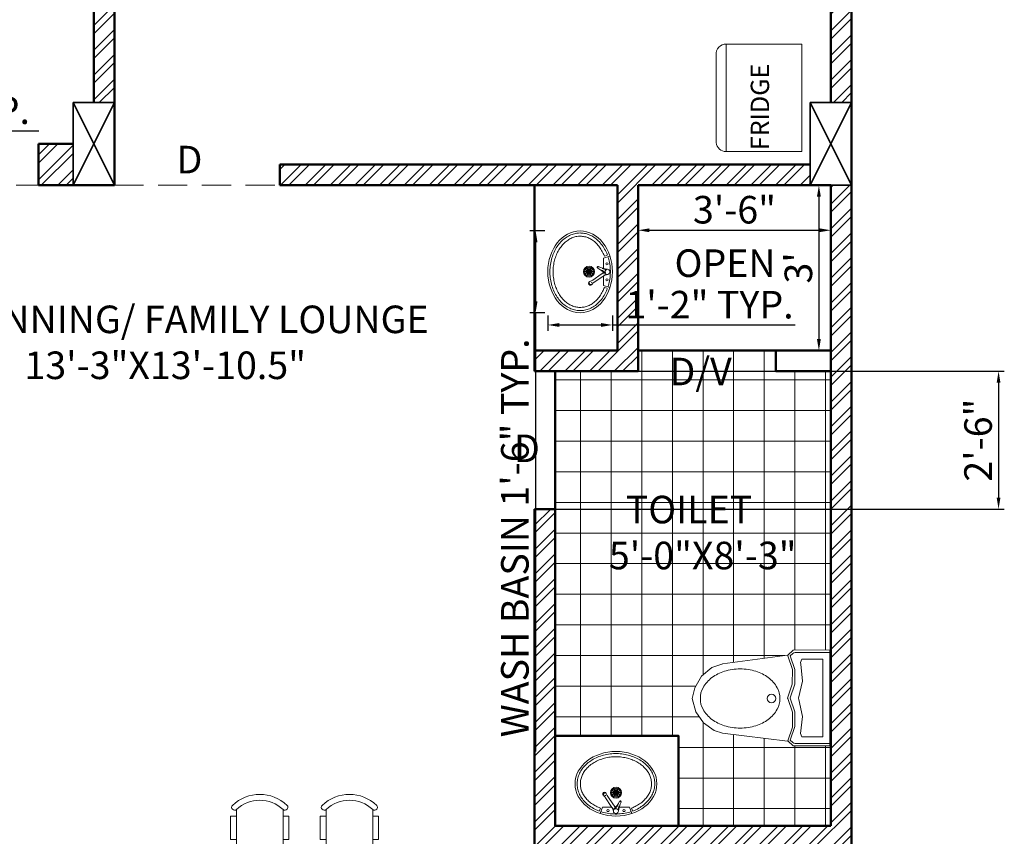
# Model space of a CAD drawing. Units: millimetres. Extents: x 67033 to 68301, y 155969 to 157209.
# Tile 5 of 17: x 67226 to 67441, y 156800 to 156978. Entities that reach past the tile are written whole.
import ezdxf

# ---------------------------------------------------------------- set-up
doc = ezdxf.new("R2010")
doc.units = ezdxf.units.MM
doc.linetypes.add('HIDDEN', pattern=[9.525, 6.35, -3.175])
for name, color, linetype, lineweight in [('A-ANNO-DIMS', 2, 'Continuous', 18), ('A-ANNO-TEXT', 7, 'Continuous', 18), ('A-AREA-IDEN', 3, 'Continuous', 18), ('A-COLS', 3, 'Continuous', 35), ('A-EQPM', 8, 'Continuous', 18), ('A-FLOR-FIXT', 9, 'Continuous', 18), ('A-FLOR-OVHD', 1, 'HIDDEN', 18), ('A-FLOR-PATT', 252, 'Continuous', 13), ('A-FURN', 8, 'Continuous', 18), ('A-WALL', 7, 'Continuous', 50), ('A-WALL-PATT', 8, 'Continuous', 13)]:
    doc.layers.add(name, color=color, linetype=linetype, lineweight=lineweight)
doc.styles.get("Standard").update_dxf_attribs({"font": 'arial.ttf'})
doc.dimstyles.new('ISO-25', dxfattribs={"dimtxt": 6, "dimasz": 2.5, "dimexe": 1.25, "dimexo": 0.625, "dimtad": 1, "dimdec": 0, "dimlunit": 3, "dimtxsty": 'Standard', "dimcen": 2.5, "dimadec": 0, "dimazin": 0, "dimtfac": 1, "dimtdec": 0, "dimtmove": 0, "dimatfit": 3, "dimfxl": 1, "dimarcsym": 0})

# ---------------------------------------------------------------- blocks, each defined once
blk = doc.blocks.new('A$C1AC47749')
for p, q in [((0.1857, 0.4482), (0.192, 0.4291)), ((0.1907, 0.471), (0.2068, 0.4222)), ((0.4293, 0.471), (0.4132, 0.4222)), ((0.4343, 0.4482), (0.428, 0.4291)), ((0.2068, 0.4222), (0.2842, 0.4222)), ((0.328, 0.4053), (0.3724, 0.3403)), ((0.4132, 0.4222), (0.3413, 0.4222)), ((0.3893, 0.3519), (0.3454, 0.4162))]:
    blk.add_line(p, q)
for centre, radius in [((0.2494, 0.448), 0.00831), ((0.3706, 0.448), 0.00831), ((0.3092, 0.3122), 0.0419), ((0.3092, 0.3122), 0.0344), ((0.3092, 0.3122), 0.00537)]:
    blk.add_circle(centre, radius)
for centre, radius, start, end in [((0.0375, 0.4868), 0.255, 336.13579, 352.27707), ((0.31, 0.4499), 0.02, 316.21432, 172.27707), ((0.4278, 0.4728), 0.1, 191.02619, 214.5133), ((0.2768, 0.381), 0.00664, 156.13579, 332.3556), ((0.2783, 0.3821), 0.00491, 187.76508, 270.74833), ((0.5085, 0.2596), 0.255, 136.21432, 152.3556), ((0.2063, 0.4499), 0.0866, 334.5047, 356.00596), ((0.3092, 0.4498), 0.0162, 192.84427, 306.07085), ((0.3746, 0.3688), 0.0866, 132.48544, 153.98669), ((0.1778, 0.1242), 0.3257, 64.69826, 65.8021), ((0.2456, 0.3486), 0.1, 34.51324, 47.88111), ((0.299, 0.3998), 0.0293, 33.00691, 56.74915), ((0.3603, 0.4414), 0.0293, 186.64626, 215.15328), ((0.29, 0.2836), 0.1, 20.01079, 34.51324), ((0.3971, 0.3226), 0.0139, 200.01079, 49.01574), ((0.3943, 0.3268), 0.00759, 93.32422, 152.57703), ((0.4717, 0.4086), 0.1, 214.5133, 229.01574), ((0.397, 0.323), 0.00812, 242.55567, 44.63645), ((0.3988, 0.322), 0.00965, 313.38275, 23.63796)]:
    blk.add_arc(centre, radius, start, end)
for centre, major_axis, ratio in [((0.31, 0.2449), (-0.31, 0), 0.790323), ((0.2894, 0.3122), (0.0145, 0), 0.137964), ((0.292, 0.3221), (0.0126, -0.0072), 0.137964), ((0.292, 0.3022), (0.0126, 0.0072), 0.137964), ((0.2993, 0.3294), (0.0072, -0.0126), 0.137964), ((0.2993, 0.295), (0.0072, 0.0126), 0.137964), ((0.3092, 0.332), (0, -0.0145), 0.137964), ((0.3092, 0.2923), (0, 0.0145), 0.137964), ((0.3192, 0.3294), (-0.0072, -0.0126), 0.137964), ((0.3192, 0.295), (-0.0072, 0.0126), 0.137964), ((0.3264, 0.3221), (-0.0126, -0.0072), 0.137964), ((0.3264, 0.3022), (-0.0126, 0.0072), 0.137964), ((0.3291, 0.3122), (-0.0145, 0), 0.137964)]:
    blk.add_ellipse(centre, major_axis=major_axis, ratio=ratio)
for points, knots in [([(0.1844, 0.4522), (0.1793, 0.4504), (0.1743, 0.4484), (0.1546, 0.44), (0.1406, 0.4328), (0.1143, 0.4165), (0.102, 0.4076), (0.0797, 0.3882), (0.0697, 0.3778), (0.052, 0.3558), (0.0443, 0.3443), (0.0317, 0.3205), (0.0267, 0.3083), (0.0194, 0.2833), (0.0171, 0.2706), (0.0158, 0.2536), (0.0156, 0.2492), (0.0156, 0.2449), (0.0156, 0.2369), (0.0162, 0.229), (0.019, 0.2084), (0.022, 0.1958), (0.0309, 0.1711), (0.0366, 0.159), (0.0508, 0.1357), (0.0591, 0.1244), (0.0781, 0.1031), (0.0888, 0.0931), (0.1123, 0.0746), (0.1251, 0.066), (0.1524, 0.0508), (0.1669, 0.0441), (0.1972, 0.0327), (0.213, 0.028), (0.2454, 0.0207), (0.262, 0.0182), (0.2956, 0.0154), (0.3125, 0.0152), (0.3462, 0.0169), (0.3629, 0.0189), (0.3956, 0.0251), (0.4117, 0.0293), (0.4426, 0.0397), (0.4574, 0.046), (0.4855, 0.0604), (0.4987, 0.0685), (0.5232, 0.0863), (0.5344, 0.096), (0.5545, 0.1167), (0.5635, 0.1277), (0.5788, 0.1506), (0.5851, 0.1625), (0.5953, 0.187), (0.599, 0.1995), (0.6037, 0.2248), (0.6047, 0.2375), (0.6039, 0.263), (0.6021, 0.2758), (0.5959, 0.3009), (0.5914, 0.3133), (0.5798, 0.3373), (0.5727, 0.349), (0.556, 0.3714), (0.5464, 0.382), (0.5249, 0.402), (0.5131, 0.4113), (0.4875, 0.4282), (0.4738, 0.4358), (0.4516, 0.446), (0.4437, 0.4492), (0.4356, 0.4522)], [5.14883, 5.14883, 5.14883, 5.14883, 5.205467, 5.205467, 5.375452, 5.375452, 5.545437, 5.545437, 5.715422, 5.715422, 5.885408, 5.885408, 6.055393, 6.055393, 6.225378, 6.225378, 6.283185, 6.283185, 6.283185, 6.389094, 6.389094, 6.559079, 6.559079, 6.729064, 6.729064, 6.89905, 6.89905, 7.069035, 7.069035, 7.23902, 7.23902, 7.409005, 7.409005, 7.578991, 7.578991, 7.748976, 7.748976, 7.918961, 7.918961, 8.088947, 8.088947, 8.258932, 8.258932, 8.428917, 8.428917, 8.598902, 8.598902, 8.768888, 8.768888, 8.938873, 8.938873, 9.108858, 9.108858, 9.278843, 9.278843, 9.448829, 9.448829, 9.618814, 9.618814, 9.788799, 9.788799, 9.958784, 9.958784, 10.12877, 10.12877, 10.298755, 10.298755, 10.46874, 10.46874, 10.559126, 10.559126, 10.559126, 10.559126]), ([(0.4244, 0.4561), (0.4209, 0.4573), (0.4174, 0.4584), (0.3981, 0.4641), (0.3818, 0.4677), (0.3487, 0.4726), (0.3319, 0.474), (0.2982, 0.4744), (0.2813, 0.4735), (0.248, 0.4694), (0.2315, 0.4663), (0.2088, 0.4603), (0.2022, 0.4583), (0.1956, 0.4561)], [4.3173628, 4.3173628, 4.3173628, 4.3173628, 4.3555402, 4.3555402, 4.5255255, 4.5255255, 4.6955107, 4.6955107, 4.865496, 4.865496, 5.0354813, 5.0354813, 5.1074083, 5.1074083, 5.1074083, 5.1074083]), ([(0.192, 0.4291), (0.1828, 0.4257), (0.1739, 0.4219), (0.1529, 0.4117), (0.1412, 0.4049), (0.1193, 0.3901), (0.1093, 0.382), (0.0911, 0.3649), (0.0829, 0.3558), (0.0687, 0.3371), (0.0626, 0.3273), (0.0526, 0.3074), (0.0487, 0.2972), (0.043, 0.2767), (0.0411, 0.2663), (0.0401, 0.2522), (0.04, 0.2486), (0.04, 0.2449), (0.04, 0.2369), (0.0406, 0.229), (0.0435, 0.2107), (0.0461, 0.2004), (0.0536, 0.1801), (0.0584, 0.1701), (0.0702, 0.1506), (0.0771, 0.1411), (0.093, 0.1229), (0.1019, 0.1142), (0.1217, 0.098), (0.1324, 0.0904), (0.1556, 0.0766), (0.168, 0.0704), (0.1939, 0.0596), (0.2075, 0.055), (0.2356, 0.0476), (0.2501, 0.0447), (0.2794, 0.0409), (0.2943, 0.0399), (0.3242, 0.0398), (0.3391, 0.0408), (0.3685, 0.0445), (0.3829, 0.0472), (0.4111, 0.0546), (0.4247, 0.0591), (0.4508, 0.0698), (0.4632, 0.076), (0.4864, 0.0897), (0.4973, 0.0972), (0.5171, 0.1134), (0.5262, 0.122), (0.5422, 0.1401), (0.5492, 0.1496), (0.561, 0.1691), (0.5659, 0.1791), (0.5736, 0.1994), (0.5763, 0.2097), (0.5797, 0.2304), (0.5803, 0.2408), (0.5794, 0.2617), (0.5779, 0.272), (0.5728, 0.2926), (0.5692, 0.3029), (0.5599, 0.3229), (0.5541, 0.3327), (0.5405, 0.3517), (0.5327, 0.3609), (0.5151, 0.3783), (0.5053, 0.3865), (0.4839, 0.4017), (0.4724, 0.4087), (0.4499, 0.4202), (0.4392, 0.4249), (0.428, 0.4291)], [5.15203, 5.15203, 5.15203, 5.15203, 5.262547, 5.262547, 5.423175, 5.423175, 5.583803, 5.583803, 5.744431, 5.744431, 5.90506, 5.90506, 6.065688, 6.065688, 6.226316, 6.226316, 6.283185, 6.283185, 6.283185, 6.405631, 6.405631, 6.566259, 6.566259, 6.726887, 6.726887, 6.887515, 6.887515, 7.048143, 7.048143, 7.208772, 7.208772, 7.3694, 7.3694, 7.530028, 7.530028, 7.690656, 7.690656, 7.851284, 7.851284, 8.011912, 8.011912, 8.172541, 8.172541, 8.333169, 8.333169, 8.493797, 8.493797, 8.654425, 8.654425, 8.815053, 8.815053, 8.975681, 8.975681, 9.13631, 9.13631, 9.296938, 9.296938, 9.457566, 9.457566, 9.618194, 9.618194, 9.778822, 9.778822, 9.93945, 9.93945, 10.100079, 10.100079, 10.260707, 10.260707, 10.421335, 10.421335, 10.555929, 10.555929, 10.555929, 10.555929])]:
    blk.add_open_spline(points, degree=3, knots=knots)
blk = doc.blocks.new('A$C09D638C3')
for p, q in [((0, 0.7166), (0.0008, 0.5263)), ((0.2504, 0.7166), (0, 0.7166)), ((0.0137, 0.7166), (0.0137, 0.5365)), ((0.048, 0.6794), (0.048, 0.5712)), ((0.2504, 0.6794), (0.048, 0.6794)), ((0.2504, 0.7166), (0.5, 0.7166)), ((0.2504, 0.6794), (0.4528, 0.6794)), ((0.4528, 0.6794), (0.4528, 0.5712)), ((0.4871, 0.7166), (0.4871, 0.5365)), ((0.5, 0.7166), (0.5, 0.5263)), ((0.048, 0.5712), (0.0652, 0.5632)), ((0.0733, 0.5655), (0.0652, 0.5632)), ((0.1631, 0.5735), (0.0733, 0.5655)), ((0.2504, 0.5527), (0.1631, 0.5735)), ((0.3462, 0.574), (0.2582, 0.5558)), ((0.4356, 0.5632), (0.3462, 0.574)), ((0.4528, 0.5712), (0.4356, 0.5632)), ((0.0008, 0.5263), (0.0274, 0.4973)), ((0.0137, 0.5365), (0.015, 0.5295)), ((0.015, 0.5295), (0.0189, 0.5233)), ((0.0189, 0.5233), (0.019, 0.5232)), ((0.019, 0.5232), (0.0309, 0.5105)), ((0.102, 0.522), (0.0297, 0.4985)), ((0.1021, 0.5341), (0.0309, 0.5105)), ((0.1786, 0.5213), (0.102, 0.522)), ((0.1781, 0.5339), (0.1021, 0.5341)), ((0.2494, 0.5098), (0.1781, 0.5339)), ((0.2504, 0.4965), (0.1786, 0.5213)), ((0.2582, 0.5558), (0.2504, 0.5527)), ((0.3224, 0.5339), (0.2514, 0.5098)), ((0.3248, 0.5217), (0.2527, 0.4977)), ((0.3984, 0.5342), (0.3224, 0.5339)), ((0.4014, 0.5216), (0.3248, 0.5217)), ((0.47, 0.5105), (0.3984, 0.5342)), ((0.4734, 0.4973), (0.4014, 0.5216)), ((0.4818, 0.5232), (0.47, 0.5105)), ((0.5, 0.5263), (0.4734, 0.4973)), ((0.4818, 0.5232), (0.4857, 0.5293)), ((0.4857, 0.5293), (0.4871, 0.5363)), ((0.4871, 0.5363), (0.4871, 0.5365)), ((0.0271, 0.4967), (0.072, 0.1582)), ((0.0297, 0.4985), (0.0274, 0.4973)), ((0.2527, 0.4977), (0.2504, 0.4965)), ((0.4758, 0.4967), (0.4334, 0.1581)), ((0.0718, 0.1596), (0.0917, 0.1021)), ((0.4201, 0.1144), (0.4334, 0.1581)), ((0.3799, 0.0583), (0.4201, 0.1144)), ((0.0917, 0.1021), (0.1359, 0.0488)), ((0.3218, 0.0186), (0.3799, 0.0583)), ((0.1359, 0.0488), (0.1968, 0.0131)), ((0.1968, 0.0131), (0.2526, 0)), ((0.2528, 0), (0.3218, 0.0186))]:
    blk.add_line(p, q)
blk.add_circle((0.2527, 0.4124), 0.0222)
for centre, radius, start, end in [((0.2776, 0.2962), 0.1668, 118.8748, 143.2661), ((0.2513, 0.3471), 0.1095, 89.1493, 119.7298), ((0.2546, 0.3471), 0.1095, 60.2702, 90.8507), ((0.2283, 0.2962), 0.1668, 36.7339, 61.1252), ((0.3216, 0.265), 0.2207, 143.6094, 162.4475), ((0.1843, 0.265), 0.2207, 17.5525, 36.3906), ((0.3937, 0.2468), 0.295, 163.3175, 179.5076), ((0.1122, 0.2468), 0.295, 0.4924, 16.6825), ((0.3937, 0.2519), 0.295, 180.4924, 196.6825), ((0.1122, 0.2519), 0.295, 343.3175, 359.5076), ((0.3216, 0.2338), 0.2207, 197.5525, 216.3906), ((0.1843, 0.2338), 0.2207, 323.6094, 342.4475), ((0.2776, 0.2026), 0.1668, 216.7339, 241.1252), ((0.2283, 0.2026), 0.1668, 298.8748, 323.2661), ((0.2513, 0.1516), 0.1095, 240.2702, 270.8507), ((0.2546, 0.1516), 0.1095, 269.1493, 299.7298)]:
    blk.add_arc(centre, radius, start, end)
blk = doc.blocks.new('table dining')
for p, q in [((67480.1, 156784.21), (67480.1, 156775.8)), ((67490.26, 156775.8), (67490.26, 156784.21)), ((67499.62, 156784.21), (67499.62, 156775.8)), ((67509.78, 156775.8), (67509.78, 156784.21)), ((67480.1, 156782.75), (67478.83, 156782.75)), ((67478.83, 156777.67), (67478.83, 156782.75)), ((67490.26, 156782.75), (67491.53, 156782.75)), ((67491.53, 156777.67), (67491.53, 156782.75)), ((67499.62, 156782.75), (67498.35, 156782.75)), ((67498.35, 156777.67), (67498.35, 156782.75)), ((67509.78, 156782.75), (67511.05, 156782.75)), ((67511.05, 156777.67), (67511.05, 156782.75)), ((67480.1, 156777.67), (67478.83, 156777.67)), ((67490.26, 156777.67), (67491.53, 156777.67)), ((67499.62, 156777.67), (67498.35, 156777.67)), ((67509.78, 156777.67), (67511.05, 156777.67)), ((67476.09, 156751.17), (67476.09, 156775.04)), ((67476.85, 156775.8), (67513.43, 156775.8)), ((67514.19, 156751.17), (67514.19, 156775.04)), ((67469.03, 156768.18), (67469.03, 156769.45)), ((67474.11, 156769.45), (67469.03, 156769.45)), ((67474.11, 156768.18), (67474.11, 156769.45)), ((67516.16, 156768.18), (67516.16, 156769.45)), ((67516.16, 156769.45), (67521.24, 156769.45)), ((67521.24, 156768.18), (67521.24, 156769.45)), ((67476.09, 156768.18), (67467.57, 156768.18)), ((67514.19, 156768.18), (67522.71, 156768.18)), ((67467.57, 156758.02), (67476.09, 156758.02)), ((67469.03, 156758.02), (67469.03, 156756.75)), ((67474.11, 156758.02), (67474.11, 156756.75)), ((67522.71, 156758.02), (67514.19, 156758.02)), ((67516.16, 156758.02), (67516.16, 156756.75)), ((67521.24, 156758.02), (67521.24, 156756.75)), ((67474.11, 156756.75), (67469.03, 156756.75)), ((67516.16, 156756.75), (67521.24, 156756.75)), ((67476.85, 156750.4), (67513.43, 156750.4))]:
    blk.add_line(p, q)
for centre, radius, start, end in [((67485.18, 156778.87), 8.64, 46.4394, 133.5606), ((67485.18, 156778.87), 7.37, 46.4394, 133.5606), ((67504.7, 156778.87), 8.64, 46.4394, 133.5606), ((67504.7, 156778.87), 7.37, 46.4394, 133.5606), ((67479.7, 156784.71), 0.637, 138.3417, 308.7795), ((67490.66, 156784.71), 0.637, 231.2205, 41.6583), ((67499.22, 156784.71), 0.637, 138.3417, 308.7795), ((67510.18, 156784.71), 0.637, 231.2205, 41.6583), ((67476.85, 156775.04), 0.762, 90, 180), ((67513.43, 156775.04), 0.762, 0, 90), ((67472.91, 156763.1), 8.64, 136.4394, 223.5606), ((67467.07, 156768.58), 0.637, 321.2205, 131.6583), ((67523.2, 156768.58), 0.637, 48.3417, 218.7795), ((67517.37, 156763.1), 8.64, 316.4394, 43.5606), ((67472.91, 156763.1), 7.37, 136.4394, 223.5606), ((67517.37, 156763.1), 7.37, 316.4394, 43.5606), ((67467.07, 156757.62), 0.637, 228.3417, 38.7795), ((67523.2, 156757.62), 0.637, 141.2205, 311.6583), ((67476.85, 156751.17), 0.762, 180, 270), ((67513.43, 156751.17), 0.762, 270, 0)]:
    blk.add_arc(centre, radius, start, end)
blk = doc.blocks.new('*D27')
at = {"layer": 'A-ANNO-DIMS', "color": 0, "lineweight": -2, "transparency": 16777216}
for p, q in [((67360.94, 156935.93), (67360.94, 156930.94)), ((67402.94, 156935.93), (67402.94, 156930.94)), ((67363.44, 156932.19), (67400.44, 156932.19))]:
    blk.add_line(p, q, dxfattribs=at)
at = {"layer": 'A-ANNO-DIMS', "color": 0, "transparency": 16777216}
for points in [[(67363.44, 156932.6), (67363.44, 156931.77), (67360.94, 156932.19)], [(67400.44, 156932.6), (67400.44, 156931.77), (67402.94, 156932.19)]]:
    blk.add_solid(points, dxfattribs=at)
at = {"layer": 'Defpoints', "color": 0, "transparency": 16777216}
for p in [(67360.94, 156936.55), (67402.94, 156936.55), (67402.94, 156932.19)]:
    blk.add_point(p, dxfattribs=at)
at = {"layer": 'A-ANNO-DIMS', "color": 0, "transparency": 16777216, "insert": (67381.94, 156935.88), "char_height": 6, "attachment_point": 5}
blk.add_mtext('3\'-6"', dxfattribs=at)
blk = doc.blocks.new('*D28')
at = {"layer": 'A-ANNO-DIMS', "color": 0, "lineweight": -2, "transparency": 16777216}
for p, q in [((67397.44, 156941.99), (67401.57, 156941.99)), ((67400.32, 156939.49), (67400.32, 156908.49)), ((67397.44, 156905.99), (67401.57, 156905.99))]:
    blk.add_line(p, q, dxfattribs=at)
at = {"layer": 'A-ANNO-DIMS', "color": 0, "transparency": 16777216}
for points in [[(67399.9, 156939.49), (67400.74, 156939.49), (67400.32, 156941.99)], [(67399.9, 156908.49), (67400.74, 156908.49), (67400.32, 156905.99)]]:
    blk.add_solid(points, dxfattribs=at)
at = {"layer": 'Defpoints', "color": 0, "transparency": 16777216}
for p in [(67396.81, 156941.99), (67396.81, 156905.99), (67400.32, 156905.99)]:
    blk.add_point(p, dxfattribs=at)
at = {"layer": 'A-ANNO-DIMS', "color": 0, "transparency": 16777216, "insert": (67396.63, 156923.99), "char_height": 6, "attachment_point": 5, "rotation": 90}
blk.add_mtext("3'", dxfattribs=at)
blk = doc.blocks.new('COLUMN-230x460')
for p, q in [((0.44, 17.99), (9.44, -0.01)), ((9.44, 17.99), (0.44, -0.01))]:
    blk.add_line(p, q)
blk.add_lwpolyline([(0.44, 17.99), (9.44, 17.99), (9.44, -0.01), (0.44, -0.01)], close=True)
blk = doc.blocks.new('FRIDGE')
for p, q in [((18.68, 23.4), (2.13, 23.4)), ((2.2, 23.4), (2.2, 0)), ((18.68, 0), (18.68, 23.4)), ((0.01, 21.05), (0.01, 1.99)), ((2.13, 0), (18.68, 0))]:
    blk.add_line(p, q)
for centre, start, end in [((2.17, 21.23), 89.0957, 184.6304), ((2.17, 2.17), 184.6304, 270.9043)]:
    blk.add_arc(centre, 2.17, start, end)
blk = doc.blocks.new('*D53')
at = {"layer": 'A-ANNO-DIMS', "color": 0, "lineweight": -2, "transparency": 16777216}
for p, q in [((67340.69, 156932.04), (67337.39, 156932.04)), ((67338.64, 156929.54), (67338.64, 156916.74)), ((67340.69, 156914.24), (67337.39, 156914.24)), ((67338.64, 156914.24), (67338.64, 156818.71))]:
    blk.add_line(p, q, dxfattribs=at)
at = {"layer": 'A-ANNO-DIMS', "color": 0, "transparency": 16777216}
for points in [[(67338.22, 156929.54), (67339.06, 156929.54), (67338.64, 156932.04)], [(67338.22, 156916.74), (67339.06, 156916.74), (67338.64, 156914.24)]]:
    blk.add_solid(points, dxfattribs=at)
at = {"layer": 'Defpoints', "color": 0, "transparency": 16777216}
for p in [(67341.31, 156932.04), (67338.64, 156914.24), (67341.31, 156914.24)]:
    blk.add_point(p, dxfattribs=at)
at = {"layer": 'A-ANNO-DIMS', "color": 0, "transparency": 16777216, "insert": (67334.91, 156865.22), "char_height": 6, "attachment_point": 5, "rotation": 90}
blk.add_mtext('WASH BASIN 1\'-6" TYP.', dxfattribs=at)
blk = doc.blocks.new('*D54')
at = {"layer": 'A-ANNO-DIMS', "color": 0, "lineweight": -2, "transparency": 16777216}
for p, q in [((67341.31, 156913.61), (67341.31, 156910.32)), ((67355.38, 156913.61), (67355.38, 156910.32)), ((67343.81, 156911.57), (67352.88, 156911.57)), ((67355.38, 156911.57), (67395.14, 156911.57))]:
    blk.add_line(p, q, dxfattribs=at)
at = {"layer": 'A-ANNO-DIMS', "color": 0, "transparency": 16777216}
for points in [[(67343.81, 156911.98), (67343.81, 156911.15), (67341.31, 156911.57)], [(67352.88, 156911.98), (67352.88, 156911.15), (67355.38, 156911.57)]]:
    blk.add_solid(points, dxfattribs=at)
at = {"layer": 'Defpoints', "color": 0, "transparency": 16777216}
for p in [(67341.31, 156914.24), (67355.38, 156914.24), (67355.38, 156911.57)]:
    blk.add_point(p, dxfattribs=at)
at = {"layer": 'A-ANNO-DIMS', "color": 0, "transparency": 16777216, "insert": (67376.51, 156915.21), "char_height": 6, "attachment_point": 5}
blk.add_mtext('1\'-2" TYP.', dxfattribs=at)
blk = doc.blocks.new('*D77')
at = {"layer": 'A-ANNO-DIMS', "color": 0, "lineweight": -2, "transparency": 16777216}
for p, q in [((67121.85, 156949.49), (67121.85, 156955.1)), ((67155.1, 156949.49), (67155.1, 156955.1)), ((67124.35, 156953.85), (67152.6, 156953.85)), ((67155.1, 156953.85), (67230.5, 156953.85))]:
    blk.add_line(p, q, dxfattribs=at)
at = {"layer": 'A-ANNO-DIMS', "color": 0, "transparency": 16777216}
for points in [[(67124.35, 156954.27), (67124.35, 156953.43), (67121.85, 156953.85)], [(67152.6, 156954.27), (67152.6, 156953.43), (67155.1, 156953.85)]]:
    blk.add_solid(points, dxfattribs=at)
at = {"layer": 'Defpoints', "color": 0, "transparency": 16777216}
for p in [(67155.1, 156953.85), (67121.85, 156948.86), (67155.1, 156948.86)]:
    blk.add_point(p, dxfattribs=at)
at = {"layer": 'A-ANNO-DIMS', "color": 0, "transparency": 16777216, "insert": (67194.05, 156957.54), "char_height": 6, "attachment_point": 5}
blk.add_mtext('TV UNIT 2\'-9" TYP.', dxfattribs=at)
blk = doc.blocks.new('*D93')
at = {"layer": 'A-ANNO-DIMS', "color": 0, "lineweight": -2, "transparency": 16777216}
for p, q in [((67242.44, 156960.62), (67242.44, 157174.24)), ((67246.94, 156960.62), (67246.94, 157174.24)), ((67239.94, 157172.99), (67237.44, 157172.99)), ((67242.44, 157172.99), (67246.94, 157172.99)), ((67249.44, 157172.99), (67283.12, 157172.99))]:
    blk.add_line(p, q, dxfattribs=at)
at = {"layer": 'A-ANNO-DIMS', "color": 0, "transparency": 16777216}
for points in [[(67239.94, 157173.41), (67239.94, 157172.58), (67242.44, 157172.99)], [(67249.44, 157173.41), (67249.44, 157172.58), (67246.94, 157172.99)]]:
    blk.add_solid(points, dxfattribs=at)
at = {"layer": 'Defpoints', "color": 0, "transparency": 16777216}
for p in [(67246.94, 157172.99), (67242.44, 156959.99), (67246.94, 156959.99)]:
    blk.add_point(p, dxfattribs=at)
at = {"layer": 'A-ANNO-DIMS', "color": 0, "transparency": 16777216, "insert": (67267.53, 157176.72), "char_height": 6, "attachment_point": 5}
blk.add_mtext('0\'-4 1/2"', dxfattribs=at)
blk = doc.blocks.new('*D95')
at = {"layer": 'A-ANNO-DIMS', "color": 0, "lineweight": -2, "transparency": 16777216}
for p, q in [((67339.06, 156901.49), (67440.69, 156901.49)), ((67439.44, 156898.99), (67439.44, 156873.99)), ((67339.06, 156871.49), (67440.69, 156871.49))]:
    blk.add_line(p, q, dxfattribs=at)
at = {"layer": 'A-ANNO-DIMS', "color": 0, "transparency": 16777216}
for points in [[(67439.02, 156898.99), (67439.85, 156898.99), (67439.44, 156901.49)], [(67439.02, 156873.99), (67439.85, 156873.99), (67439.44, 156871.49)]]:
    blk.add_solid(points, dxfattribs=at)
at = {"layer": 'Defpoints', "color": 0, "transparency": 16777216}
for p in [(67338.44, 156901.49), (67338.44, 156871.49), (67439.44, 156871.49)]:
    blk.add_point(p, dxfattribs=at)
at = {"layer": 'A-ANNO-DIMS', "color": 0, "transparency": 16777216, "insert": (67435.75, 156886.49), "char_height": 6, "attachment_point": 5, "rotation": 90}
blk.add_mtext('2\'-6"', dxfattribs=at)

msp = doc.modelspace()

# ---------------------------------------------------------------- hatches: boundary and pattern name
at = {"layer": 'A-FLOR-PATT'}
h = msp.add_hatch(dxfattribs=at)
h.set_pattern_fill('NET', color=256, scale=2.1)
h.paths.add_polyline_path([(67402.94, 156901.49), (67390.94, 156901.49), (67390.94, 156905.99), (67360.94, 156905.99), (67360.94, 156901.49), (67342.94, 156901.49), (67342.94, 156871.49), (67342.94, 156822.09), (67369.78, 156822.09), (67369.78, 156802.49), (67402.94, 156802.49)])
h.paths.add_polyline_path([(67393.55, 156839.69), (67394.74, 156840.78), (67402.7, 156840.81), (67402.7, 156830.35), (67402.7, 156819.92), (67394.74, 156819.92), (67393.66, 156820.91), (67379.35, 156822.7), (67377.53, 156823.26), (67375.19, 156824.94), (67373.53, 156827.36), (67372.75, 156830.25), (67373.29, 156832.59), (67374.79, 156835.13), (67377.01, 156836.98), (67379.42, 156837.81)], flags=16)
h.paths.add_polyline_path([(67383.17, 156836.69, -0.07076), (67386.6, 156836.17, -0.082382), (67389.29, 156834.8, -0.106831), (67391.23, 156832.58, -0.13423), (67391.83, 156830.24, -0.13423), (67391.23, 156827.91, -0.106831), (67389.29, 156825.68, -0.082382), (67386.6, 156824.32, -0.07076), (67383.17, 156823.8, -0.07076), (67379.74, 156824.32, -0.082382), (67377.04, 156825.68, -0.106831), (67375.11, 156827.91, -0.13423), (67374.51, 156830.24, -0.13423), (67375.11, 156832.58, -0.106831), (67377.04, 156834.8, -0.082382), (67379.74, 156836.17, -0.07076)], flags=0)
h.paths.add_polyline_path([(67393.51, 156830.38), (67393.55, 156830.25), (67393.5, 156830.35)], flags=0)
h.paths.add_polyline_path([(67394.62, 156840.03), (67394.61, 156840.02), (67394.08, 156839.53), (67395.07, 156836.55), (67395.06, 156833.37), (67394.04, 156830.35), (67395.06, 156827.34), (67395.07, 156824.16), (67394.08, 156821.17), (67394.61, 156820.68), (67394.87, 156820.52), (67395.16, 156820.46), (67395.17, 156820.46), (67395.16, 156820.46), (67394.87, 156820.52), (67394.61, 156820.68), (67394.08, 156821.17), (67395.07, 156824.16), (67395.06, 156827.34), (67394.04, 156830.35), (67395.06, 156833.37), (67395.07, 156836.55), (67394.08, 156839.53), (67394.62, 156840.03)], flags=0)
h.paths.add_polyline_path([(67396.62, 156838.81), (67401.14, 156838.81), (67401.14, 156830.35), (67401.14, 156821.89), (67396.62, 156821.89), (67396.29, 156822.61), (67396.73, 156826.35), (67395.98, 156830.02), (67395.85, 156830.35), (67396.71, 156834), (67396.38, 156837.75), (67396.29, 156838.09)], flags=0)
h.paths.add_polyline_path([(67390.91, 156830.25, -1), (67389.06, 156830.25, -1)], flags=0)
h.paths.add_polyline_path([(67362.63, 156895.05), (67384.26, 156895.05), (67384.26, 156907.42), (67362.63, 156907.42)], flags=9)
h.paths.add_polyline_path([(67352.75, 156854.97), (67394.72, 156854.97), (67394.72, 156877.36), (67352.75, 156877.36)], flags=24)
at = {"layer": 'A-WALL-PATT'}
h = msp.add_hatch(dxfattribs=at)
h.set_pattern_fill('ANSI32', color=256, scale=0.4)
h.paths.add_polyline_path([(67246.94, 157064.99), (67242.44, 157064.99), (67242.44, 156959.99), (67246.94, 156959.99)])
h = msp.add_hatch(dxfattribs=at)
h.set_pattern_fill('ANSI32', color=256, scale=0.4)
h.paths.add_polyline_path([(67407.44, 157061.19), (67402.94, 157061.19), (67402.94, 156959.99), (67407.44, 156959.99)])
h = msp.add_hatch(dxfattribs=at)
h.set_pattern_fill('ANSI32', color=256, scale=0.4)
h.paths.add_polyline_path([(67237.94, 156950.99), (67230.44, 156950.99), (67230.44, 156941.99), (67237.94, 156941.99)])
h = msp.add_hatch(dxfattribs=at)
h.set_pattern_fill('ANSI32', color=256, scale=0.4)
h.paths.add_polyline_path([(67398.44, 156946.49), (67282.94, 156946.49), (67282.94, 156941.99), (67356.44, 156941.99), (67356.44, 156905.99), (67338.44, 156905.99), (67338.44, 156901.49), (67360.94, 156901.49), (67360.94, 156941.99), (67398.44, 156941.99)])
h = msp.add_hatch(dxfattribs=at)
h.set_pattern_fill('ANSI32', color=256, scale=0.4)
h.paths.add_polyline_path([(67407.44, 156941.99), (67402.94, 156941.99), (67402.94, 156802.49), (67342.94, 156802.49), (67342.94, 156822.09), (67342.94, 156871.49), (67338.44, 156871.49), (67338.44, 156770.99), (67236.44, 156770.99), (67236.44, 156766.49), (67338.44, 156766.49), (67338.44, 156685.49), (67342.94, 156685.49), (67342.94, 156797.99), (67402.94, 156797.99), (67402.94, 156767.19), (67407.44, 156767.19)])

# ---------------------------------------------------------------- linework, layer by layer
at = {"layer": 'A-FLOR-OVHD'}
for p, q in [((67196.98, 156941.99), (67230.44, 156941.99)), ((67246.94, 156941.99), (67282.94, 156941.99))]:
    msp.add_line(p, q, dxfattribs=at)
at = {"layer": 'A-WALL'}
for p, q in [((67407.44, 157140.99), (67407.44, 156527.99)), ((67246.94, 157082.99), (67246.94, 156941.99)), ((67242.44, 157064.99), (67242.44, 156959.99)), ((67402.94, 157061.19), (67402.94, 156959.99)), ((67230.44, 156950.99), (67230.44, 156941.99)), ((67230.44, 156950.99), (67237.94, 156950.99)), ((67282.94, 156946.49), (67398.44, 156946.49)), ((67282.94, 156946.49), (67282.94, 156941.99)), ((67230.44, 156941.99), (67246.94, 156941.99)), ((67282.94, 156941.99), (67356.44, 156941.99)), ((67338.44, 156941.99), (67338.44, 156901.49)), ((67356.44, 156941.99), (67356.44, 156905.99)), ((67360.94, 156941.99), (67360.94, 156901.49)), ((67360.94, 156941.99), (67402.94, 156941.99)), ((67402.94, 156941.99), (67402.94, 156802.49)), ((67338.44, 156905.99), (67356.44, 156905.99)), ((67390.94, 156905.99), (67360.94, 156905.99)), ((67390.94, 156905.99), (67390.94, 156901.49)), ((67390.94, 156905.99), (67402.94, 156905.99)), ((67338.44, 156901.49), (67360.94, 156901.49)), ((67342.94, 156871.49), (67342.94, 156901.49)), ((67390.94, 156901.49), (67402.94, 156901.49)), ((67338.44, 156871.49), (67342.94, 156871.49)), ((67338.44, 156871.49), (67338.44, 156770.99)), ((67342.94, 156871.49), (67342.94, 156802.49)), ((67342.94, 156802.49), (67402.94, 156802.49))]:
    msp.add_line(p, q, dxfattribs=at)
msp.add_lwpolyline([(67342.94, 156822.09), (67369.78, 156822.09), (67369.78, 156802.49), (67342.94, 156802.49)], close=True, dxfattribs=at)

# ---------------------------------------------------------------- block references
at = {"layer": 'A-COLS'}
for p in [(67237.5, 156942), (67398, 156942)]:
    msp.add_blockref('COLUMN-230x460', p, dxfattribs=at)
at = {"layer": 'A-EQPM'}
msp.add_blockref('FRIDGE', (67377.94, 156949.31), dxfattribs=at)
at = {"layer": 'A-FLOR-FIXT'}
for name, p, xscale, yscale, zscale, rotation in [('A$C1AC47749', (67341.31, 156932.04), 28.71035709425155, 28.71035709425155, 28.71035709425155, 270), ('A$C09D638C3', (67372.75, 156840.81), 41.79230271587537, 41.79230271587537, 41.79230271587537, 270), ('A$C1AC47749', (67365.04, 156818.71), 28.71035709425095, 28.71035709425095, 28.71035709425095, 180)]:
    msp.add_blockref(name, p, dxfattribs=dict(at, xscale=xscale, yscale=yscale, zscale=zscale, rotation=rotation))
at = {"layer": 'A-FURN'}
msp.add_blockref('table dining', (-206.59, 21.85), dxfattribs=at)

# ---------------------------------------------------------------- texts
at = {"layer": 'A-ANNO-TEXT', "insert": (67385.48, 156945.96), "char_height": 4, "attachment_point": 1, "rotation": 90}
msp.add_mtext_dynamic_manual_height_columns('   FRIDGE', width=46.8836, gutter_width=12.5, heights=[0], dxfattribs=at)
at = {"layer": 'A-ANNO-TEXT', "char_height": 6, "attachment_point": 1}
for s, insert in [('   D', (67254.98, 156950.57)), ('  D/V', (67364.13, 156904.43)), ('   D', (67328.45, 156887.7))]:
    msp.add_mtext_dynamic_manual_height_columns(s, width=19.5287, gutter_width=12.5, heights=[0], dxfattribs=dict(at, insert=insert))
at = {"layer": 'A-AREA-IDEN', "char_height": 6, "attachment_point": 1}
for s, width, insert in [('        OPEN', 46.8836, (67354.23, 156928.02)), ('  DINNING/ FAMILY LOUNGE\\P         13\'-3"X13\'-10.5"', 118.0294, (67210.86, 156915.79)), ('  TOILET                         5\'-0"X8\'-3"', 43.4182, (67354.6, 156874.38))]:
    msp.add_mtext_dynamic_manual_height_columns(s, width=width, gutter_width=12.5, heights=[0], dxfattribs=dict(at, insert=insert))

# ---------------------------------------------------------------- dimensions: what is measured, and where the dimension line sits
at = {"layer": 'A-ANNO-DIMS'}
for base, p1, p2, override, picture, middle in [((67246.94, 157172.99), (67242.44, 156959.99), (67246.94, 156959.99), {"dimdec": 1, "dimlfac": 1, "dimrnd": 0, "dimzin": 1, "dimdsep": 46, "dimlunit": 4, "dimfrac": 2}, '*D93', (67267.53, 157176.72)), ((67402.94, 156932.19), (67360.94, 156936.55), (67402.94, 156936.55), {"dimclrd": 0, "dimclre": 0, "dimclrt": 0}, '*D27', (67381.94, 156935.88))]:
    dim = msp.add_linear_dim(base=base, p1=p1, p2=p2, dimstyle='ISO-25', override=override, dxfattribs=at)
    dim.commit()
    dim.dimension.update_dxf_attribs({"geometry": picture, "text_midpoint": middle})
for base, p1, p2, text, picture, middle in [((67155.1043, 156953.8516), (67121.8549, 156948.8642), (67155.1043, 156948.8642), 'TV UNIT <> TYP.', '*D77', (67194.0534, 156957.54)), ((67355.38, 156911.57), (67341.31, 156914.24), (67355.38, 156914.24), '<> TYP.', '*D54', (67376.51, 156915.21))]:
    dim = msp.add_linear_dim(base=base, p1=p1, p2=p2, text=text, dimstyle='ISO-25', override={"dimdec": 1, "dimrnd": 0, "dimzin": 1, "dimlunit": 4, "dimfrac": 2}, dxfattribs=at)
    dim.commit()
    dim.dimension.update_dxf_attribs({"geometry": picture, "text_midpoint": middle})
for base, p1, p2, override, picture, middle in [((67400.32, 156905.99), (67396.81, 156941.99), (67396.81, 156905.99), {"dimclrd": 0, "dimclre": 0, "dimclrt": 0}, '*D28', (67396.63, 156923.99)), ((67439.44, 156871.49), (67338.44, 156901.49), (67338.44, 156871.49), {"dimdec": 1, "dimlfac": 1, "dimrnd": 0, "dimzin": 1, "dimdsep": 46, "dimlunit": 4, "dimfrac": 2}, '*D95', (67435.75, 156886.49))]:
    dim = msp.add_linear_dim(base=base, p1=p1, p2=p2, angle=90, dimstyle='ISO-25', override=override, dxfattribs=at)
    dim.commit()
    dim.dimension.update_dxf_attribs({"geometry": picture, "text_midpoint": middle})
dim = msp.add_linear_dim(base=(67338.64, 156914.24), p1=(67341.31, 156932.04), p2=(67341.31, 156914.24), angle=270, text='WASH BASIN <> TYP.', dimstyle='ISO-25', override={"dimdec": 1, "dimrnd": 0, "dimzin": 1, "dimlunit": 4, "dimfrac": 2}, dxfattribs=at)
dim.commit()
dim.dimension.update_dxf_attribs({"geometry": '*D53', "text_midpoint": (67334.91, 156865.22)})

doc.saveas('drawing.dxf')
